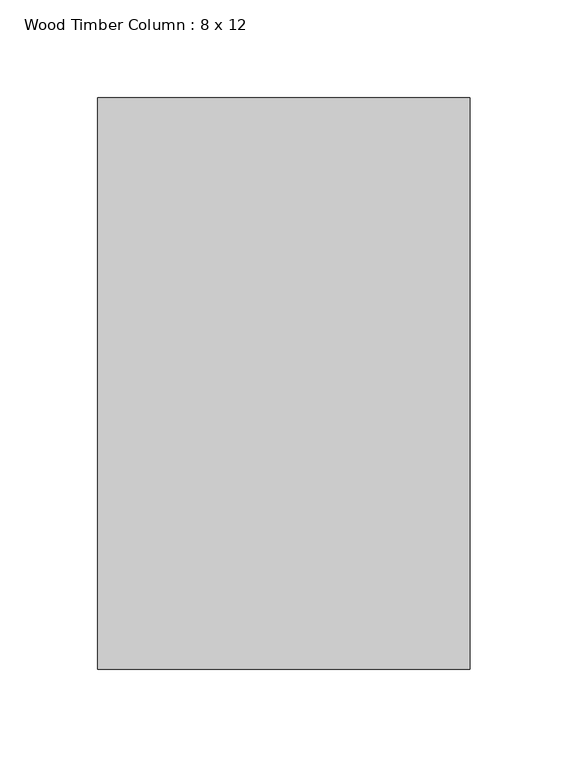
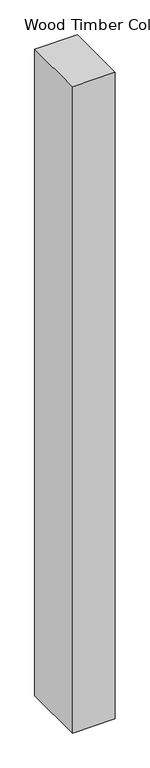
"""IFC4 building model written with IfcOpenShell, lengths in millimetres: column geometry, Wood Timber Column : 8 x 12."""

from ifc_helpers import new_model, si_unit, frame, origin, place, context, project, spatial, polyline, outline, extrude, source, transform, mapped, element, save


def wood_timber_column_8_x_12_853526f8(model_context):
    return source(origin(), model_context, "Body", "SweptSolid", [
        extrude(outline(polyline([(95.25, -146.05), (-95.25, -146.05), (-95.25, 146.05), (95.25, 146.05), (95.25, -146.05)])), frame((0.0, 0.0, 7844.0883406), z_axis=(0.0, 0.0, 1.0), x_axis=(1.0, 0.0, 0.0)), (0.0, 0.0, 1.0), 3048.0),
    ])


if __name__ == "__main__":
    model = new_model("IFC4")
    model_context = context("Model", 3, world=origin())
    ifc_project = project(units=[si_unit("LENGTHUNIT", "METRE", prefix="MILLI")], contexts=[model_context])
    site = spatial("IfcSite", under=ifc_project)
    building = spatial("IfcBuilding", under=site)
    placement = place(None, origin())
    wood_timber_column_8_x_12_shape = wood_timber_column_8_x_12_853526f8(model_context)
    element("IfcColumn", 1, ObjectType="Wood Timber Column : 8 x 12", at=placement, inside=building, context=model_context, shape_type="MappedRepresentation", body=[
        mapped(wood_timber_column_8_x_12_shape, transform((0.0, 0.0, 0.0), x_axis=(1.0, 0.0, 0.0), y_axis=(0.0, 1.0, 0.0), z_axis=(0.0, 0.0, 1.0))),
    ])
    save(model, "model.ifc")

# Revit data of these elements
# Type "Wood Timber Column : 8 x 12"
#   Assembly Code = "B1010200"
#   Depth = 0' - 11 1/2"
#   Width = 0' - 7 1/2"
#   Material = Softwood, Lumber
# Element 1 (IfcColumn, "Wood Timber Column : 8 x 12")
#   Materials on its faces: "Softwood, Lumber"
# Materials
#   "Softwood, Lumber": class "Wood", colour RGB 223 192 134, transparency 0, Description = "Pinus Echinata", Cost = 0
